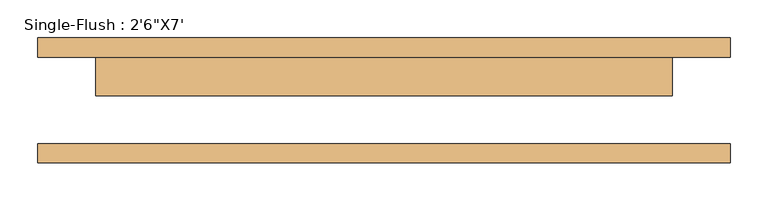
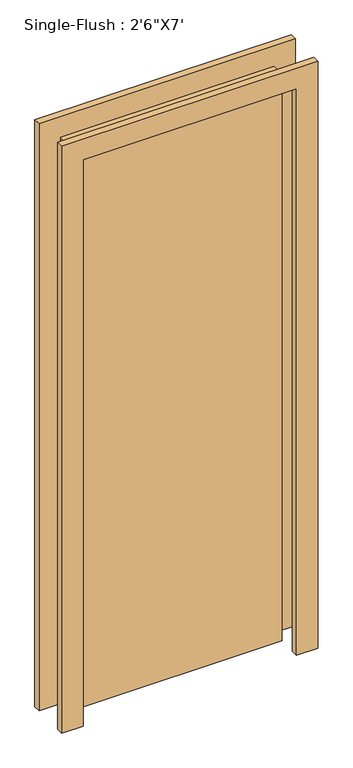
"""IFC4 building model written with IfcOpenShell, lengths in millimetres: door geometry."""

from ifc_helpers import new_model, si_unit, frame, origin, origin_with_axes, place, context, project, spatial, polyline, outline, extrude, source, transform, mapped, element, save


def door_214872d5(model_context):
    return source(origin(), model_context, "Body", "SweptSolid", [
        extrude(outline(polyline([(2209.8, -457.2), (0.0, -457.2), (0.0, -381.0), (2133.6, -381.0), (2133.6, 381.0), (0.0, 381.0), (0.0, 457.2), (2209.8, 457.2), (2209.8, -457.2)])), frame((0.0, 57.15, 0.0), z_axis=(0.0, 1.0, 0.0), x_axis=(0.0, 0.0, 1.0)), (0.0, 0.0, 1.0), 25.4),
        extrude(outline(polyline([(2209.8, 457.2), (2209.8, -457.2), (0.0, -457.2), (0.0, -381.0), (2133.6, -381.0), (2133.6, 381.0), (0.0, 381.0), (0.0, 457.2), (2209.8, 457.2)])), frame((0.0, -82.55, 0.0), z_axis=(0.0, 1.0, 0.0), x_axis=(0.0, 0.0, 1.0)), (0.0, 0.0, 1.0), 25.4),
        extrude(outline(polyline([(381.0, 6.35), (-381.0, 6.35), (-381.0, 57.15), (381.0, 57.15), (381.0, 6.35)])), origin_with_axes(), (0.0, 0.0, 1.0), 2133.6),
    ])


if __name__ == "__main__":
    model = new_model("IFC4")
    model_context = context("Model", 3, world=origin())
    ifc_project = project(units=[si_unit("LENGTHUNIT", "METRE", prefix="MILLI")], contexts=[model_context])
    site = spatial("IfcSite", under=ifc_project)
    building = spatial("IfcBuilding", under=site)
    placement = place(None, origin())
    door_shape = door_214872d5(model_context)
    element("IfcDoor", 1, ObjectType="Single-Flush : 2'6\"X7'", at=placement, inside=building, context=model_context, shape_type="MappedRepresentation", body=[
        mapped(door_shape, transform((0.0, 0.0, 0.0), x_axis=(1.0, 0.0, 0.0), y_axis=(0.0, 1.0, 0.0), z_axis=(0.0, 0.0, 1.0))),
    ])
    save(model, "model.ifc")

# Revit data of these elements
# Type "Single-Flush : 2'6\"X7'"
#   Type Mark = "13"
#   Construction Type Id = "MDOOR"
#   Assembly Code = "C1020"
#   Analytic Construction = "Metal"
#   Thickness = 0' - 2"
#   Heat Transfer Coefficient (U) = 0.651978 BTU/(h·ft²·°F)
#   Height = 7' - 0"
#   Trim Projection Ext = 0' - 1"
#   Trim Projection Int = 0' - 1"
#   Trim Width = 0' - 3"
#   Width = 2' - 6"
#   Define Thermal Properties by = 1
#   Door Material = Door - Panel
#   Frame Material = Door - Frame
#   Visual Light Transmittance = 0
#   Solar Heat Gain Coefficient = 0
#   Function = (empty or 0)
#   Wall Closure = (empty or 0)
# Element 1 (IfcDoor, "Single-Flush : 2'6\"X7'")
#   Materials on its faces: "Door - Frame", "Door - Panel"
# Materials
#   "Door - Panel": class "Wood", colour RGB 210 159 95, transparency 0, Cost = 0
#   "Door - Frame": colour RGB 118 70 51, transparency 0, Cost = 0
